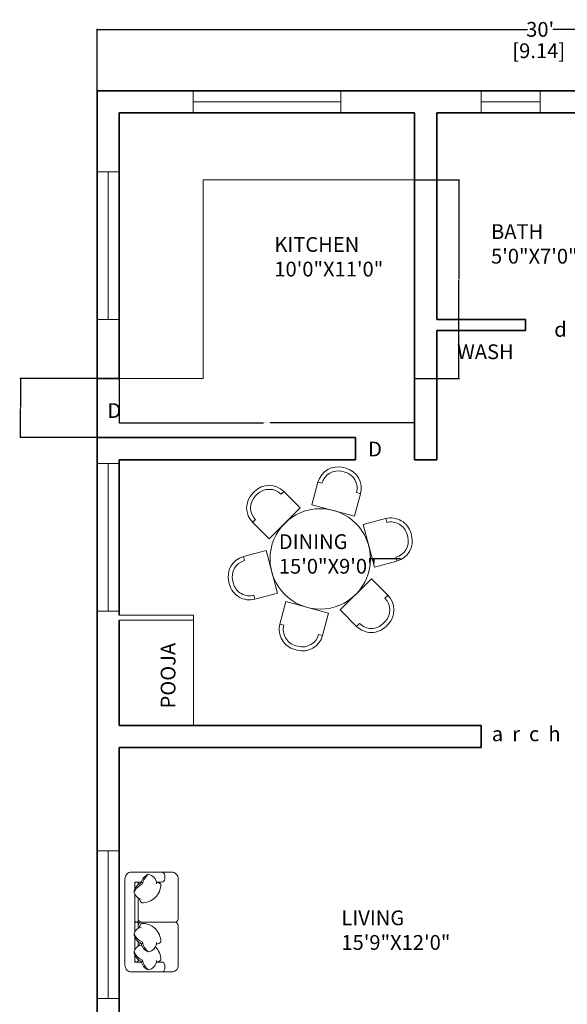
# Model space of a CAD drawing. Units: inches. Extents: x -43 to 1296, y -568 to 542.
# Tile 2 of 14: x -3 to 220, y -365 to 36. Entities that reach past the tile are written whole.
import ezdxf

# ---------------------------------------------------------------- set-up
doc = ezdxf.new("R2010")
doc.units = ezdxf.units.IN
doc.header["$MEASUREMENT"] = 0
for name, color, linetype, lineweight in [('A-ANNO-DIMS', 2, 'Continuous', 18), ('A-ANNO-TEXT', 7, 'Continuous', 18), ('A-AREA-IDEN', 7, 'Continuous', 18), ('A-FLOR-CASE', 9, 'Continuous', 18), ('A-FURN', 8, 'Continuous', 13), ('A-GLAZ', 6, 'Continuous', 18), ('A-WALL', 7, 'Continuous', 35)]:
    doc.layers.add(name, color=color, linetype=linetype, lineweight=lineweight)
doc.styles.get("Standard").update_dxf_attribs({"font": 'arial.ttf'})
doc.dimstyles.get("Standard").update_dxf_attribs({"dimtxt": 0.18, "dimasz": 0.18, "dimexe": 0.18, "dimexo": 0.0625, "dimgap": 0.09, "dimtad": 0, "dimtih": 1, "dimtoh": 1, "dimdec": 0, "dimzin": 0, "dimdsep": 46, "dimlunit": 3, "dimtxsty": 'Standard', "dimcen": 0.09, "dimadec": 0, "dimazin": 0, "dimtfac": 1, "dimtdec": 0, "dimtofl": 0, "dimtmove": 0, "dimatfit": 3, "dimfxl": 1, "dimtolj": 1, "dimtzin": 0, "dimarcsym": 0})

# ---------------------------------------------------------------- blocks, each defined once
blk = doc.blocks.new('*D1')
at = {"layer": 'A-ANNO-DIMS', "color": 0, "lineweight": -2, "transparency": 16777216}
for p, q in [((28.84, 6.72), (28.84, 31.8)), ((29.02, 31.62), (203.66, 31.62)), ((388.66, 31.62), (214.02, 31.62)), ((388.84, 6.72), (388.84, 31.8))]:
    blk.add_line(p, q, dxfattribs=at)
at = {"layer": 'A-ANNO-DIMS', "color": 0, "transparency": 16777216}
for points in [[(29.02, 31.65), (29.02, 31.59), (28.84, 31.62)], [(388.66, 31.65), (388.66, 31.59), (388.84, 31.62)]]:
    blk.add_solid(points, dxfattribs=at)
at = {"layer": 'Defpoints', "color": 0, "transparency": 16777216}
for p in [(388.84, 31.62), (28.84, 6.66), (388.84, 6.66)]:
    blk.add_point(p, dxfattribs=at)
at = {"layer": 'A-ANNO-DIMS', "color": 0, "transparency": 16777216, "insert": (208.84, 31.62), "char_height": 6, "attachment_point": 5}
blk.add_mtext("\\A1;30'", dxfattribs=at)
blk = doc.blocks.new('TABLE-ROUND-6-SEAT')
for p, q in [((47.37, 72.71), (46.43, 72.96)), ((47.79, 74.28), (46.85, 74.53)), ((36.48, 68.55), (34.04, 59.43)), ((38.14, 68.18), (36.5, 68.62)), ((10.67, 64.84), (9.98, 64.15)), ((21.48, 63.69), (22.64, 64.84)), ((22.64, 64.84), (29.31, 58.16)), ((52.2, 64.34), (53.78, 63.91)), ((11.82, 63.69), (11.13, 63)), ((53.78, 63.91), (51.33, 54.8)), ((29.31, 58.16), (16.65, 45.5)), ((51.33, 54.8), (34.04, 59.43)), ((11.13, 53.43), (9.93, 52.23)), ((9.98, 52.18), (16.65, 45.5)), ((63.91, 53.78), (54.8, 51.33)), ((64.42, 52.15), (63.98, 53.79)), ((59.43, 34.04), (54.8, 51.33)), ((72.96, 46.43), (72.71, 47.37)), ((74.53, 46.85), (74.28, 47.79)), ((6.27, 38.33), (15.38, 40.77)), ((15.38, 40.77), (20.02, 23.48)), ((6.69, 36.76), (6.27, 38.33)), ((68.55, 36.49), (59.43, 34.04)), ((68.13, 38.06), (68.55, 36.49)), ((1.86, 28.39), (2.11, 27.44)), ((45.5, 16.65), (58.16, 29.31)), ((64.84, 22.64), (58.16, 29.31)), ((0.28, 27.97), (0.54, 27.02)), ((10.39, 22.66), (10.83, 21.02)), ((10.9, 21.04), (20.02, 23.48)), ((21.04, 10.9), (23.48, 20.02)), ((23.48, 20.02), (40.77, 15.38)), ((63.69, 21.38), (64.89, 22.58)), ((52.18, 9.98), (45.5, 16.65)), ((38.33, 6.27), (40.77, 15.38)), ((22.61, 10.48), (21.04, 10.9)), ((53.33, 11.13), (52.18, 9.98)), ((62.99, 11.13), (63.69, 11.82)), ((64.15, 9.98), (64.84, 10.67)), ((36.67, 6.64), (38.31, 6.2)), ((27.02, 0.54), (27.97, 0.28)), ((27.44, 2.11), (28.39, 1.86))]:
    blk.add_line(p, q)
blk.add_circle((37.41, 37.41), 20.4)
for centre, radius, start, end in [((44.66, 66.36), 8.46, 75, 165), ((44.66, 66.36), 6.83, 75, 165), ((45.6, 66.1), 6.83, 345, 75), ((45.6, 66.1), 8.46, 345, 75), ((15.96, 58.16), 8.46, 135, 225), ((16.65, 58.85), 8.46, 45, 135), ((16.65, 58.85), 6.83, 45, 135), ((15.96, 58.16), 6.83, 135, 225), ((66.1, 45.6), 8.46, 15, 105), ((66.1, 45.6), 6.83, 15, 105), ((66.36, 44.66), 6.83, 285, 15), ((66.36, 44.66), 8.46, 285, 15), ((8.46, 30.16), 8.46, 105, 195), ((8.46, 30.16), 6.83, 105, 195), ((8.71, 29.21), 8.46, 195, 285), ((8.71, 29.21), 6.83, 195, 285), ((58.85, 16.65), 6.83, 315, 45), ((58.85, 16.65), 8.46, 315, 45), ((29.21, 8.71), 8.46, 165, 255), ((29.21, 8.71), 6.83, 165, 255), ((58.16, 15.96), 8.46, 225, 315), ((58.16, 15.96), 6.83, 225, 315), ((30.16, 8.46), 8.46, 255, 345), ((30.16, 8.46), 6.83, 255, 345)]:
    blk.add_arc(centre, radius, start, end)
blk = doc.blocks.new('WIN-60x9')
for p, q in [((0, 60), (0, 0)), ((9, 60), (0, 60)), ((4.5, 60), (4.5, 0)), ((9, 0), (9, 60)), ((0, 0), (9, 0))]:
    blk.add_line(p, q)
blk = doc.blocks.new('VENT-24x9')
for p, q in [((0, 0), (0, 24)), ((0, 24), (9, 24)), ((4.5, 24), (4.5, 0)), ((9, 24), (9, 0)), ((9, 0), (0, 0))]:
    blk.add_line(p, q)
blk = doc.blocks.new('COUNTER-KITCHEN-L')
for p, q in [((34.04, 0), (34.04, 80.76)), ((34.04, 80.76), (120, 80.76)), ((0, 0), (34.04, 0))]:
    blk.add_line(p, q)
blk = doc.blocks.new('*D46')
at = {"layer": 'A-ANNO-DIMS', "color": 0, "lineweight": -2, "transparency": 16777216}
for p, q in [((37.84, -110.4), (37.84, -128.52)), ((157.84, -110.4), (157.84, -128.52)), ((38.02, -128.34), (96.48, -128.34)), ((157.66, -128.34), (99.21, -128.34))]:
    blk.add_line(p, q, dxfattribs=at)
at = {"layer": 'A-ANNO-DIMS', "color": 0, "transparency": 16777216}
for points in [[(38.02, -128.31), (38.02, -128.37), (37.84, -128.34)], [(157.66, -128.31), (157.66, -128.37), (157.84, -128.34)]]:
    blk.add_solid(points, dxfattribs=at)
at = {"layer": 'Defpoints', "color": 0, "transparency": 16777216}
for p in [(37.84, -110.34), (157.84, -110.34), (157.84, -128.34)]:
    blk.add_point(p, dxfattribs=at)
at = {"layer": 'A-ANNO-DIMS', "color": 0, "transparency": 16777216, "insert": (97.84, -128.34), "char_height": 0.18, "attachment_point": 5}
blk.add_mtext('\\A1;COUNTER 10\'-0" TYP.', dxfattribs=at)
blk = doc.blocks.new('*D47')
at = {"layer": 'A-ANNO-DIMS', "color": 0, "lineweight": -2, "transparency": 16777216}
for p, q in [((157.91, -29.58), (176.02, -29.58)), ((175.84, -29.76), (175.84, -69.78)), ((175.84, -110.16), (175.84, -70.14)), ((157.91, -110.34), (176.02, -110.34))]:
    blk.add_line(p, q, dxfattribs=at)
at = {"layer": 'A-ANNO-DIMS', "color": 0, "transparency": 16777216}
for points in [[(175.81, -29.76), (175.87, -29.76), (175.84, -29.58)], [(175.81, -110.16), (175.87, -110.16), (175.84, -110.34)]]:
    blk.add_solid(points, dxfattribs=at)
at = {"layer": 'Defpoints', "color": 0, "transparency": 16777216}
for p in [(157.84, -29.58), (175.84, -29.58), (157.84, -110.34)]:
    blk.add_point(p, dxfattribs=at)
at = {"layer": 'A-ANNO-DIMS', "color": 0, "transparency": 16777216, "insert": (175.84, -69.96), "char_height": 0.18, "attachment_point": 5}
blk.add_mtext('\\A1;6\'-9" TYP.', dxfattribs=at)
blk = doc.blocks.new('*D59')
at = {"layer": 'A-ANNO-DIMS', "color": 0, "lineweight": -2, "transparency": 16777216}
for p, q in [((28.78, -110.34), (-2.49, -110.34)), ((-2.31, -110.52), (-2.31, -122.16)), ((-2.31, -134.16), (-2.31, -122.52)), ((28.78, -134.34), (-2.49, -134.34))]:
    blk.add_line(p, q, dxfattribs=at)
at = {"layer": 'A-ANNO-DIMS', "color": 0, "transparency": 16777216}
for points in [[(-2.34, -110.52), (-2.28, -110.52), (-2.31, -110.34)], [(-2.34, -134.16), (-2.28, -134.16), (-2.31, -134.34)]]:
    blk.add_solid(points, dxfattribs=at)
at = {"layer": 'Defpoints', "color": 0, "transparency": 16777216}
for p in [(28.84, -110.34), (-2.31, -134.34), (28.84, -134.34)]:
    blk.add_point(p, dxfattribs=at)
at = {"layer": 'A-ANNO-DIMS', "color": 0, "transparency": 16777216, "insert": (-2.31, -122.34), "char_height": 0.18, "attachment_point": 5}
blk.add_mtext('\\A1;2\'-0"', dxfattribs=at)
blk = doc.blocks.new('*D97')
at = {"layer": 'A-ANNO-DIMS', "color": 0, "lineweight": -2, "transparency": 16777216}
for p, q in [((119.41, -183.65), (119.59, -183.65)), ((119.5, -183.74), (119.5, -183.56)), ((152.15, -183.65), (140.08, -183.65))]:
    blk.add_line(p, q, dxfattribs=at)
at = {"layer": 'A-ANNO-DIMS', "color": 0, "transparency": 16777216}
blk.add_solid([(140.08, -183.62), (140.08, -183.68), (139.9, -183.65)], dxfattribs=at)
at = {"layer": 'Defpoints', "color": 0, "transparency": 16777216}
for p in [(99.1, -183.65), (139.9, -183.65)]:
    blk.add_point(p, dxfattribs=at)
at = {"layer": 'A-ANNO-DIMS', "color": 0, "transparency": 16777216, "insert": (152.57, -183.65), "char_height": 0.18, "attachment_point": 5}
blk.add_mtext('\\A1;∅3\'-5"', dxfattribs=at)

msp = doc.modelspace()

# ---------------------------------------------------------------- linework, layer by layer
at = {"layer": 'A-FLOR-CASE'}
for p, q in [((37.84, -206.49), (68.03, -206.49)), ((68.03, -206.49), (68.03, -208.63)), ((68.03, -208.63), (37.84, -208.63)), ((68.03, -251.34), (68.03, -208.63))]:
    msp.add_line(p, q, dxfattribs=at)
at = {"layer": 'A-FURN', "ltscale": 0.03}
msp.add_lwpolyline([(61.8, -329.95, -0.414214), (60.44, -331.3, -0.414214), (61.8, -332.65), (61.8, -348.89, -0.414214), (59.09, -351.6), (42.85, -351.6, -0.414214), (40.15, -348.89), (40.15, -313.71, -0.414214), (42.85, -311), (59.09, -311, -0.414214), (61.8, -313.71), (61.8, -329.95, -0.414214), (60.44, -331.3, -0.414214), (61.8, -332.65)], format="xyb", dxfattribs=at)
at = {"layer": 'A-FURN'}
for points in [[(49.61, -311.87, 0.14773), (47.28, -315.82, 0.213343), (43.87, -319.31, 0.178662)], [(53.02, -315.74, 0.356772), (49.61, -311.87, 0.249542), (46.8, -315.38, -9.61688)], [(55.03, -311, -0.414214), (56.38, -312.36), (56.38, -313.71, -0.414214), (55.03, -315.06), (52.94, -315.06)], [(47.1, -315.27, 0.306663), (43.87, -319.31, 0.30633), (46.82, -321.95, -0.872847)], [(45.56, -316.1), (45.56, -315.6, 0.414214), (45.02, -315.06), (44.75, -315.06, 0.414214), (44.21, -315.6)], [(44.21, -315.6), (44.21, -317.91, 0.414214)], [(52.93, -315.06, -0.165541), (54.72, -315.9, -0.425989), (46.97, -323.5, -0.121523), (45.9, -321.69, 7.115464)], [(44.21, -320.16), (44.21, -330.76, 0.414214), (44.75, -331.3), (45.02, -331.3, 0.414214), (45.56, -330.76), (45.56, -321.52, 0.414214)], [(44.21, -335.15), (44.21, -331.84, -0.414214), (44.75, -331.3), (45.02, -331.3, -0.414214), (45.56, -331.84), (45.56, -333.79, -0.414214)], [(45.56, -329.95, 0.414214), (46.91, -331.3)], [(45.56, -329.95, 0.414214), (46.91, -331.3), (60.44, -331.3, 0.414214)], [(45.56, -332.65, -0.414214), (46.91, -331.3)], [(45.56, -332.65, -0.414214), (46.91, -331.3), (60.44, -331.3, -0.414214)], [(52.93, -340.25, 0.165541), (54.72, -339.41, 0.425989), (46.97, -331.82, 0.121523), (45.9, -333.62, -7.115464)], [(47.1, -340.04, -0.306663), (43.87, -336, -0.30633), (46.82, -333.37, 0.872847)], [(49.61, -343.45, -0.14773), (47.28, -339.49, -0.213343), (43.87, -336, -0.178662)], [(44.21, -342.44), (44.21, -337.4, -0.414214)], [(45.56, -339.22), (45.56, -341.08, -0.414214)], [(46.43, -339.77, 0.071865), (45.9, -340.91, -7.115464)], [(53.02, -339.57, -0.356772), (49.61, -343.45, -0.249542), (46.8, -339.93, 9.61688)], [(47.1, -347.33, -0.306663), (43.87, -343.29, -0.30633), (46.82, -340.65, 0.872847)], [(49.61, -350.74, -0.14773), (47.28, -346.78, -0.213343), (43.87, -343.29, -0.178662)], [(52.93, -347.54, 0.165541), (54.72, -346.7, 0.200231), (52.54, -341.33, 0.121523)], [(44.21, -347), (44.21, -344.69, -0.414214)], [(44.21, -344.69), (44.21, -347.54), (46.87, -347.54, -0.414214)], [(45.56, -346.5), (45.56, -347, -0.414214), (45.02, -347.54), (44.75, -347.54, -0.414214), (44.21, -347)], [(53.02, -346.86, -0.356772), (49.61, -350.74, -0.249542), (46.8, -347.22, 9.61688)], [(52.94, -347.54), (55.03, -347.54, -0.414214), (56.38, -348.89), (56.38, -350.24, -0.414214), (55.03, -351.6)]]:
    msp.add_lwpolyline(points, format="xyb", dxfattribs=at)
for points in [[(46.87, -315.06), (44.21, -315.06), (44.21, -317.91)], [(44.21, -320.16), (44.21, -335.15)], [(44.21, -337.4), (44.21, -342.44)]]:
    msp.add_lwpolyline(points, dxfattribs=at)
msp.add_lwpolyline([(44.21, -330.76), (44.21, -331.84, -0.414214), (44.75, -331.3), (45.02, -331.3, -0.414214), (45.56, -331.84), (45.56, -330.76, -0.414214), (45.02, -331.3), (44.75, -331.3, -0.414214)], format="xyb", close=True, dxfattribs=at)
at = {"layer": 'A-WALL'}
for p, q in [((28.84, 6.66), (28.84, -473.34)), ((28.84, 6.66), (388.84, 6.66)), ((37.84, -2.34), (157.84, -2.34)), ((37.84, -2.34), (37.84, -110.34)), ((157.84, -2.34), (157.84, -143.34)), ((166.84, -2.34), (166.84, -86.34)), ((166.84, -2.34), (226.84, -2.34)), ((166.84, -86.34), (202.84, -86.34)), ((202.84, -90.84), (202.84, -86.34)), ((166.84, -90.84), (202.84, -90.84)), ((166.84, -90.84), (166.84, -143.34)), ((37.84, -110.34), (28.84, -110.34)), ((37.84, -134.34), (28.84, -134.34)), ((37.84, -134.34), (133.84, -134.34)), ((133.84, -143.34), (133.84, -134.34)), ((37.84, -143.34), (133.84, -143.34)), ((37.84, -143.34), (37.84, -206.49)), ((157.84, -143.34), (166.84, -143.34)), ((37.84, -208.63), (37.84, -251.34)), ((37.84, -251.34), (184.84, -251.34)), ((184.84, -260.34), (184.84, -251.34)), ((37.84, -260.34), (184.84, -260.34)), ((37.84, -260.34), (37.84, -404.34))]:
    msp.add_line(p, q, dxfattribs=at)

# ---------------------------------------------------------------- block references
at = {"layer": 'A-FLOR-CASE'}
msp.add_blockref('COUNTER-KITCHEN-L', (37.84, -110.34), dxfattribs=at)
at = {"layer": 'A-FURN'}
msp.add_blockref('TABLE-ROUND-6-SEAT', (82.1, -221.06), dxfattribs=at)
at = {"layer": 'A-GLAZ'}
for name, p, rotation in [('WIN-60x9', (67.84, 6.66), 270.0000000000002), ('VENT-24x9', (184.84, 6.66), 269.9999999999995)]:
    msp.add_blockref(name, p, dxfattribs=dict(at, rotation=rotation))
for p in [(28.84, -86.34), (28.84, -204.92), (28.84, -362.34)]:
    msp.add_blockref('WIN-60x9', p, dxfattribs=at)

# ---------------------------------------------------------------- texts
at = {"layer": 'A-ANNO-DIMS', "insert": (197.53, 25.92), "char_height": 6, "attachment_point": 1}
msp.add_mtext_dynamic_manual_height_columns('[9.14]', width=0.2388, gutter_width=1, heights=[0], dxfattribs=at)
at = {"layer": 'A-ANNO-TEXT', "char_height": 6, "attachment_point": 1}
for s, insert in [('d', (214.55, -87.34)), ('D', (138.94, -135.99)), ('a  r  c  h', (189.19, -251.77))]:
    msp.add_mtext(s, dxfattribs=dict(at, insert=insert))
at = {"layer": 'A-ANNO-TEXT', "insert": (33.04, -120.36), "char_height": 6, "attachment_point": 1}
msp.add_mtext_dynamic_manual_height_columns('D', width=0.5519, gutter_width=1, heights=[0], dxfattribs=at)
at = {"layer": 'A-AREA-IDEN', "char_height": 6, "attachment_point": 1}
for s, insert in [('BATH\\P5\'0"X7\'0"', (188.88, -47.6)), ('KITCHEN\\P10\'0"X11\'0"', (100.85, -52.84)), ('WASH', (175.09, -96.44)), ('DINING\\P15\'0"X9\'0"', (102.69, -173.65)), ('LIVING\\P15\'9"X12\'0"', (128.1, -326.59))]:
    msp.add_mtext(s, dxfattribs=dict(at, insert=insert))
at = {"layer": 'A-AREA-IDEN', "insert": (54.7, -244.45), "char_height": 6, "attachment_point": 1, "rotation": 90}
msp.add_mtext('POOJA', dxfattribs=at)

# ---------------------------------------------------------------- dimensions: what is measured, and where the dimension line sits
at = {"layer": 'A-ANNO-DIMS'}
dim = msp.add_linear_dim(base=(388.84, 31.62), p1=(28.84, 6.66), p2=(388.84, 6.66), dimstyle='Standard', override={"dimtxt": 6, "dimclrd": 0, "dimclre": 0, "dimclrt": 0}, dxfattribs=at)
dim.commit()
dim.dimension.update_dxf_attribs({"geometry": '*D1', "text_midpoint": (208.84, 31.62)})
dim = msp.add_linear_dim(base=(175.84, -29.58), p1=(157.84, -110.34), p2=(157.84, -29.58), angle=90, text='<> TYP.', dimstyle='Standard', override={"dimdec": 1, "dimlfac": 1, "dimrnd": 0, "dimzin": 1, "dimdsep": 46, "dimlunit": 4, "dimfrac": 2}, dxfattribs=at)
dim.commit()
dim.dimension.update_dxf_attribs({"geometry": '*D47', "text_midpoint": (175.84, -69.96)})
dim = msp.add_linear_dim(base=(-2.31, -134.34), p1=(28.84, -110.34), p2=(28.84, -134.34), angle=90, dimstyle='Standard', override={"dimdec": 1, "dimlfac": 1, "dimrnd": 0, "dimzin": 1, "dimdsep": 46, "dimlunit": 4, "dimfrac": 2}, dxfattribs=at)
dim.commit()
dim.dimension.update_dxf_attribs({"geometry": '*D59', "text_midpoint": (-2.31, -122.34)})
dim = msp.add_linear_dim(base=(157.84, -128.34), p1=(37.84, -110.34), p2=(157.84, -110.34), text='COUNTER <> TYP.', dimstyle='Standard', override={"dimdec": 1, "dimlfac": 1, "dimrnd": 0, "dimzin": 1, "dimdsep": 46, "dimlunit": 4, "dimfrac": 2}, dxfattribs=at)
dim.commit()
dim.dimension.update_dxf_attribs({"geometry": '*D46', "text_midpoint": (97.84, -128.34)})
dim = msp.add_diameter_dim_2p(p1=(99.1, -183.65), p2=(139.9, -183.65), dimstyle='Standard', override={"dimdec": 1, "dimlfac": 1, "dimrnd": 0, "dimzin": 1, "dimdsep": 46, "dimlunit": 4, "dimfrac": 2}, dxfattribs=at)
dim.commit()
dim.dimension.update_dxf_attribs({"geometry": '*D97', "text_midpoint": (152.15, -183.65), "dimtype": 163})

doc.saveas('drawing.dxf')
